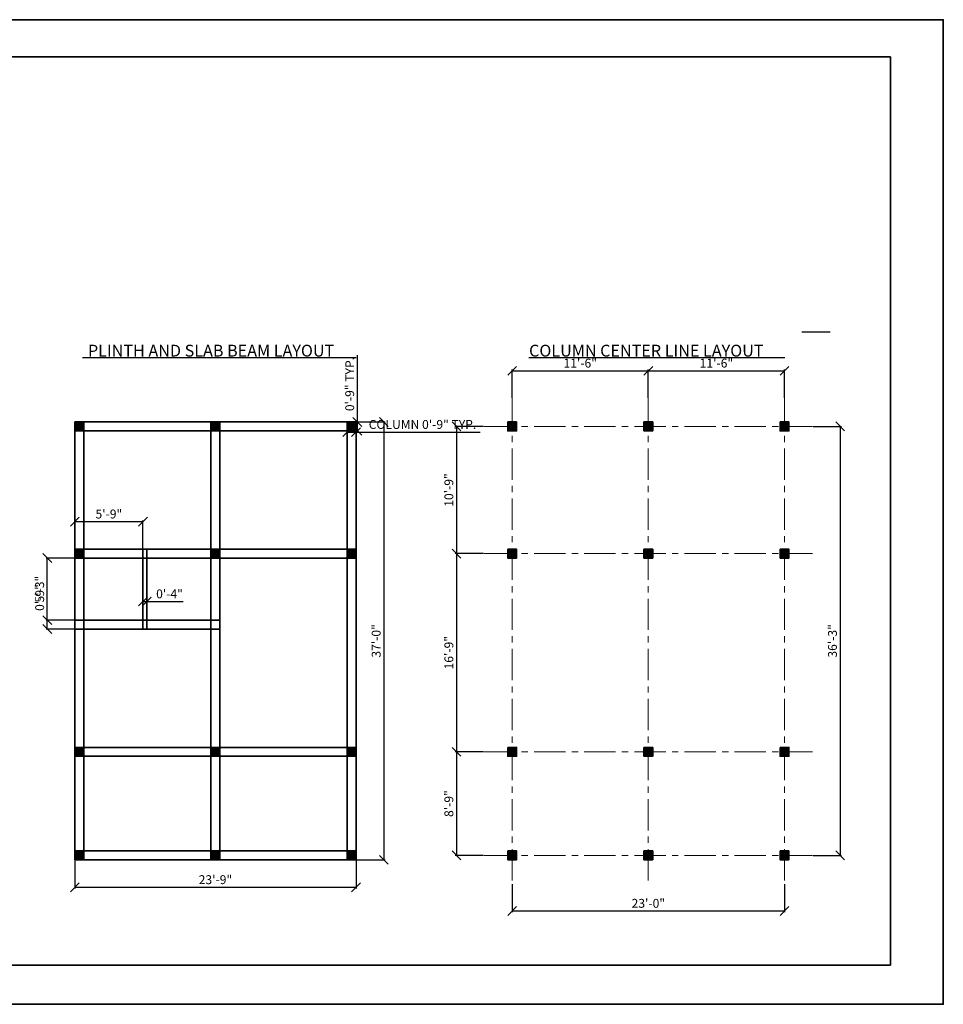
# Model space of a CAD drawing. Units: inches. Extents: x 1798 to 3594, y 1405 to 2404.
# Tile 6 of 6: x 2658 to 3594, y 1405 to 2404. Entities that reach past the tile are written whole.
import ezdxf

# ---------------------------------------------------------------- set-up
doc = ezdxf.new("R2010")
doc.units = ezdxf.units.IN
doc.linetypes.add('CENTER', pattern=[50.8, 31.75, -6.35, 6.35, -6.35])
for name, color, linetype, lineweight in [('A-ANNO-DIMS', 6, 'Continuous', 18), ('A-ANNO-TITL', 6, 'Continuous', 25), ('A-ANNO-TTLB', 7, 'Continuous', 35), ('S-BEAM', 7, 'Continuous', 35), ('S-COLS', 1, 'Continuous', 35), ('S-GRID', 8, 'CENTER', 13)]:
    doc.layers.add(name, color=color, linetype=linetype, lineweight=lineweight)
doc.styles.get("Standard").update_dxf_attribs({"font": 'arial.ttf'})
doc.dimstyles.new('ISO-25', dxfattribs={"dimtxt": 9, "dimasz": 9, "dimexe": 1.25, "dimexo": 0.625, "dimgap": 2, "dimtad": 1, "dimdec": 1, "dimlunit": 4, "dimtxsty": 'Standard', "dimblk": 'OBLIQUE', "dimcen": 2.5, "dimazin": 0, "dimtfac": 1, "dimtdec": 1, "dimtmove": 0, "dimatfit": 3, "dimfxl": 1, "dimarcsym": 0})

# ---------------------------------------------------------------- blocks, each defined once
blk = doc.blocks.new('COLUMN-9X9')
h = blk.add_hatch(color=256)
h.dxf.hatch_style = 1
h.paths.add_polyline_path([(9, 9), (0, 9), (0, 0), (9, 0)])
blk.add_lwpolyline([(0, 9), (9, 9), (9, 0), (0, 0)], close=True)
blk = doc.blocks.new('_Oblique')
at = {"color": 0, "linetype": 'ByBlock', "lineweight": -2}
blk.add_line((-0.5, -0.5), (0.5, 0.5), dxfattribs=at)
blk = doc.blocks.new('*D13')
at = {"layer": 'A-ANNO-DIMS', "color": 0, "lineweight": -2, "transparency": 16777216}
for p, q in [((2990.01, 1986.19), (2990.01, 1984.21)), ((2990.01, 1985.46), (2999.01, 1985.46)), ((2999.01, 1986.19), (2999.01, 1984.21)), ((2999.01, 1985.46), (3124.75, 1985.46))]:
    blk.add_line(p, q, dxfattribs=at)
at = {"layer": 'Defpoints', "color": 0, "transparency": 16777216}
for p in [(2990.01, 1986.81), (2999.01, 1986.81), (2999.01, 1985.46)]:
    blk.add_point(p, dxfattribs=at)
at = {"layer": 'A-ANNO-DIMS', "color": 0, "lineweight": -2, "transparency": 16777216, "xscale": 9, "yscale": 9, "zscale": 9, "rotation": 180}
blk.add_blockref('_Oblique', (2990.01, 1985.46), dxfattribs=at)
at = {"layer": 'A-ANNO-DIMS', "color": 0, "lineweight": -2, "transparency": 16777216, "xscale": 9, "yscale": 9, "zscale": 9}
blk.add_blockref('_Oblique', (2999.01, 1985.46), dxfattribs=at)
at = {"layer": 'A-ANNO-DIMS', "color": 0, "transparency": 16777216, "insert": (3066.38, 1992.12), "char_height": 9, "attachment_point": 5}
blk.add_mtext('COLUMN 0\'-9" TYP.', dxfattribs=at)
blk = doc.blocks.new('*D14')
at = {"layer": 'A-ANNO-DIMS', "color": 0, "lineweight": -2, "transparency": 16777216}
for p, q in [((3000.36, 1995.81), (3000.36, 2063.67)), ((2999.64, 1995.81), (3001.61, 1995.81)), ((3000.36, 1986.81), (3000.36, 1995.81)), ((2999.64, 1986.81), (3001.61, 1986.81))]:
    blk.add_line(p, q, dxfattribs=at)
at = {"layer": 'Defpoints', "color": 0, "transparency": 16777216}
for p in [(2999.01, 1995.81), (3000.36, 1995.81), (2999.01, 1986.81)]:
    blk.add_point(p, dxfattribs=at)
at = {"layer": 'A-ANNO-DIMS', "color": 0, "lineweight": -2, "transparency": 16777216, "xscale": 9, "yscale": 9, "zscale": 9}
for p, rotation in [((3000.36, 1995.81), 90), ((3000.36, 1986.81), 270)]:
    blk.add_blockref('_Oblique', p, dxfattribs=dict(at, rotation=rotation))
at = {"layer": 'A-ANNO-DIMS', "color": 0, "transparency": 16777216, "insert": (2993.77, 2034.24), "char_height": 9, "attachment_point": 5, "rotation": 90}
blk.add_mtext('0\'-9" TYP.', dxfattribs=at)
blk = doc.blocks.new('*D66')
at = {"layer": 'A-ANNO-DIMS', "color": 0, "lineweight": -2, "transparency": 16777216}
for p, q in [((2714.01, 1551.19), (2714.01, 1522.66)), ((2999.01, 1551.19), (2999.01, 1522.66)), ((2714.01, 1523.91), (2999.01, 1523.91))]:
    blk.add_line(p, q, dxfattribs=at)
at = {"layer": 'Defpoints', "color": 0, "transparency": 16777216}
for p in [(2714.01, 1551.81), (2999.01, 1551.81), (2999.01, 1523.91)]:
    blk.add_point(p, dxfattribs=at)
at = {"layer": 'A-ANNO-DIMS', "color": 0, "lineweight": -2, "transparency": 16777216, "xscale": 9, "yscale": 9, "zscale": 9, "rotation": 180}
blk.add_blockref('_Oblique', (2714.01, 1523.91), dxfattribs=at)
at = {"layer": 'A-ANNO-DIMS', "color": 0, "lineweight": -2, "transparency": 16777216, "xscale": 9, "yscale": 9, "zscale": 9}
blk.add_blockref('_Oblique', (2999.01, 1523.91), dxfattribs=at)
at = {"layer": 'A-ANNO-DIMS', "color": 0, "transparency": 16777216, "insert": (2856.51, 1530.51), "char_height": 9, "attachment_point": 5}
blk.add_mtext('23\'-9"', dxfattribs=at)
blk = doc.blocks.new('*D67')
at = {"layer": 'A-ANNO-DIMS', "color": 0, "lineweight": -2, "transparency": 16777216}
for p, q in [((2999.64, 1995.81), (3028.44, 1995.81)), ((3027.19, 1995.81), (3027.19, 1551.81)), ((2999.64, 1551.81), (3028.44, 1551.81))]:
    blk.add_line(p, q, dxfattribs=at)
at = {"layer": 'Defpoints', "color": 0, "transparency": 16777216}
for p in [(2999.01, 1995.81), (2999.01, 1551.81), (3027.19, 1551.81)]:
    blk.add_point(p, dxfattribs=at)
at = {"layer": 'A-ANNO-DIMS', "color": 0, "lineweight": -2, "transparency": 16777216, "xscale": 9, "yscale": 9, "zscale": 9}
for p, rotation in [((3027.19, 1995.81), 90), ((3027.19, 1551.81), 270)]:
    blk.add_blockref('_Oblique', p, dxfattribs=dict(at, rotation=rotation))
at = {"layer": 'A-ANNO-DIMS', "color": 0, "transparency": 16777216, "insert": (3020.6, 1773.81), "char_height": 9, "attachment_point": 5, "rotation": 90}
blk.add_mtext('37\'-0"', dxfattribs=at)
blk = doc.blocks.new('*D68')
at = {"layer": 'A-ANNO-DIMS', "color": 0, "lineweight": -2, "transparency": 16777216}
for p, q in [((2714.01, 1867.44), (2714.01, 1895.96)), ((2714.01, 1894.71), (2783.01, 1894.71)), ((2783.01, 1867.44), (2783.01, 1895.96))]:
    blk.add_line(p, q, dxfattribs=at)
at = {"layer": 'Defpoints', "color": 0, "transparency": 16777216}
for p in [(2783.01, 1894.71), (2714.01, 1866.81), (2783.01, 1866.81)]:
    blk.add_point(p, dxfattribs=at)
at = {"layer": 'A-ANNO-DIMS', "color": 0, "lineweight": -2, "transparency": 16777216, "xscale": 9, "yscale": 9, "zscale": 9, "rotation": 180}
blk.add_blockref('_Oblique', (2714.01, 1894.71), dxfattribs=at)
at = {"layer": 'A-ANNO-DIMS', "color": 0, "lineweight": -2, "transparency": 16777216, "xscale": 9, "yscale": 9, "zscale": 9}
blk.add_blockref('_Oblique', (2783.01, 1894.71), dxfattribs=at)
at = {"layer": 'A-ANNO-DIMS', "color": 0, "transparency": 16777216, "insert": (2748.51, 1901.31), "char_height": 9, "attachment_point": 5}
blk.add_mtext('5\'-9"', dxfattribs=at)
blk = doc.blocks.new('*D69')
at = {"layer": 'A-ANNO-DIMS', "color": 0, "lineweight": -2, "transparency": 16777216}
for p, q in [((2783.01, 1786.44), (2783.01, 1814.96)), ((2783.01, 1813.71), (2787.01, 1813.71)), ((2787.01, 1786.44), (2787.01, 1814.96)), ((2787.01, 1813.71), (2823.94, 1813.71))]:
    blk.add_line(p, q, dxfattribs=at)
at = {"layer": 'Defpoints', "color": 0, "transparency": 16777216}
for p in [(2787.01, 1813.71), (2783.01, 1785.81), (2787.01, 1785.81)]:
    blk.add_point(p, dxfattribs=at)
at = {"layer": 'A-ANNO-DIMS', "color": 0, "lineweight": -2, "transparency": 16777216, "xscale": 9, "yscale": 9, "zscale": 9, "rotation": 180}
blk.add_blockref('_Oblique', (2783.01, 1813.71), dxfattribs=at)
at = {"layer": 'A-ANNO-DIMS', "color": 0, "lineweight": -2, "transparency": 16777216, "xscale": 9, "yscale": 9, "zscale": 9}
blk.add_blockref('_Oblique', (2787.01, 1813.71), dxfattribs=at)
at = {"layer": 'A-ANNO-DIMS', "color": 0, "transparency": 16777216, "insert": (2809.98, 1820.31), "char_height": 9, "attachment_point": 5}
blk.add_mtext('0\'-4"', dxfattribs=at)
blk = doc.blocks.new('*D70')
at = {"layer": 'A-ANNO-DIMS', "color": 0, "lineweight": -2, "transparency": 16777216}
for p, q in [((2713.39, 1857.81), (2684.86, 1857.81)), ((2686.11, 1794.81), (2686.11, 1857.81)), ((2713.39, 1794.81), (2684.86, 1794.81))]:
    blk.add_line(p, q, dxfattribs=at)
at = {"layer": 'Defpoints', "color": 0, "transparency": 16777216}
for p in [(2686.11, 1857.81), (2714.01, 1857.81), (2714.01, 1794.81)]:
    blk.add_point(p, dxfattribs=at)
at = {"layer": 'A-ANNO-DIMS', "color": 0, "lineweight": -2, "transparency": 16777216, "xscale": 9, "yscale": 9, "zscale": 9}
for p, rotation in [((2686.11, 1857.81), 90), ((2686.11, 1794.81), 270)]:
    blk.add_blockref('_Oblique', p, dxfattribs=dict(at, rotation=rotation))
at = {"layer": 'A-ANNO-DIMS', "color": 0, "transparency": 16777216, "insert": (2679.51, 1826.31), "char_height": 9, "attachment_point": 5, "rotation": 90}
blk.add_mtext('5\'-3"', dxfattribs=at)
blk = doc.blocks.new('*D71')
at = {"layer": 'A-ANNO-DIMS', "color": 0, "lineweight": -2, "transparency": 16777216}
for p, q in [((2686.11, 1794.81), (2686.11, 1831.74)), ((2713.39, 1794.81), (2684.86, 1794.81)), ((2686.11, 1785.81), (2686.11, 1794.81)), ((2713.39, 1785.81), (2684.86, 1785.81))]:
    blk.add_line(p, q, dxfattribs=at)
at = {"layer": 'Defpoints', "color": 0, "transparency": 16777216}
for p in [(2686.11, 1794.81), (2714.01, 1794.81), (2714.01, 1785.81)]:
    blk.add_point(p, dxfattribs=at)
at = {"layer": 'A-ANNO-DIMS', "color": 0, "lineweight": -2, "transparency": 16777216, "xscale": 9, "yscale": 9, "zscale": 9}
for p, rotation in [((2686.11, 1794.81), 90), ((2686.11, 1785.81), 270)]:
    blk.add_blockref('_Oblique', p, dxfattribs=dict(at, rotation=rotation))
at = {"layer": 'A-ANNO-DIMS', "color": 0, "transparency": 16777216, "insert": (2679.52, 1817.77), "char_height": 9, "attachment_point": 5, "rotation": 90}
blk.add_mtext('0\'-9"', dxfattribs=at)
blk = doc.blocks.new('*D72')
at = {"layer": 'A-ANNO-DIMS', "color": 0, "lineweight": -2, "transparency": 16777216}
for p, q in [((3157.27, 2020.44), (3157.27, 2048.96)), ((3157.27, 2047.71), (3295.27, 2047.71)), ((3295.27, 2020.44), (3295.27, 2048.96))]:
    blk.add_line(p, q, dxfattribs=at)
at = {"layer": 'Defpoints', "color": 0, "transparency": 16777216}
for p in [(3295.27, 2047.71), (3157.27, 2019.81), (3295.27, 2019.81)]:
    blk.add_point(p, dxfattribs=at)
at = {"layer": 'A-ANNO-DIMS', "color": 0, "lineweight": -2, "transparency": 16777216, "xscale": 9, "yscale": 9, "zscale": 9, "rotation": 180}
blk.add_blockref('_Oblique', (3157.27, 2047.71), dxfattribs=at)
at = {"layer": 'A-ANNO-DIMS', "color": 0, "lineweight": -2, "transparency": 16777216, "xscale": 9, "yscale": 9, "zscale": 9}
blk.add_blockref('_Oblique', (3295.27, 2047.71), dxfattribs=at)
at = {"layer": 'A-ANNO-DIMS', "color": 0, "transparency": 16777216, "insert": (3226.27, 2054.31), "char_height": 9, "attachment_point": 5}
blk.add_mtext('11\'-6"', dxfattribs=at)
blk = doc.blocks.new('*D73')
at = {"layer": 'A-ANNO-DIMS', "color": 0, "lineweight": -2, "transparency": 16777216}
for p, q in [((3295.27, 2020.44), (3295.27, 2048.96)), ((3295.27, 2047.71), (3433.27, 2047.71)), ((3433.27, 2020.44), (3433.27, 2048.96))]:
    blk.add_line(p, q, dxfattribs=at)
at = {"layer": 'Defpoints', "color": 0, "transparency": 16777216}
for p in [(3433.27, 2047.71), (3295.27, 2019.81), (3433.27, 2019.81)]:
    blk.add_point(p, dxfattribs=at)
at = {"layer": 'A-ANNO-DIMS', "color": 0, "lineweight": -2, "transparency": 16777216, "xscale": 9, "yscale": 9, "zscale": 9, "rotation": 180}
blk.add_blockref('_Oblique', (3295.27, 2047.71), dxfattribs=at)
at = {"layer": 'A-ANNO-DIMS', "color": 0, "lineweight": -2, "transparency": 16777216, "xscale": 9, "yscale": 9, "zscale": 9}
blk.add_blockref('_Oblique', (3433.27, 2047.71), dxfattribs=at)
at = {"layer": 'A-ANNO-DIMS', "color": 0, "transparency": 16777216, "insert": (3364.27, 2054.31), "char_height": 9, "attachment_point": 5}
blk.add_mtext('11\'-6"', dxfattribs=at)
blk = doc.blocks.new('*D74')
at = {"layer": 'A-ANNO-DIMS', "color": 0, "lineweight": -2, "transparency": 16777216}
for p, q in [((3157.27, 1527.19), (3157.27, 1498.66)), ((3433.27, 1527.19), (3433.27, 1498.66)), ((3157.27, 1499.91), (3433.27, 1499.91))]:
    blk.add_line(p, q, dxfattribs=at)
at = {"layer": 'Defpoints', "color": 0, "transparency": 16777216}
for p in [(3157.27, 1527.81), (3433.27, 1527.81), (3433.27, 1499.91)]:
    blk.add_point(p, dxfattribs=at)
at = {"layer": 'A-ANNO-DIMS', "color": 0, "lineweight": -2, "transparency": 16777216, "xscale": 9, "yscale": 9, "zscale": 9, "rotation": 180}
blk.add_blockref('_Oblique', (3157.27, 1499.91), dxfattribs=at)
at = {"layer": 'A-ANNO-DIMS', "color": 0, "lineweight": -2, "transparency": 16777216, "xscale": 9, "yscale": 9, "zscale": 9}
blk.add_blockref('_Oblique', (3433.27, 1499.91), dxfattribs=at)
at = {"layer": 'A-ANNO-DIMS', "color": 0, "transparency": 16777216, "insert": (3295.27, 1506.51), "char_height": 9, "attachment_point": 5}
blk.add_mtext('23\'-0"', dxfattribs=at)
blk = doc.blocks.new('*D75')
at = {"layer": 'A-ANNO-DIMS', "color": 0, "lineweight": -2, "transparency": 16777216}
for p, q in [((3128.14, 1991.31), (3099.62, 1991.31)), ((3100.87, 1991.31), (3100.87, 1862.31)), ((3128.14, 1862.31), (3099.62, 1862.31))]:
    blk.add_line(p, q, dxfattribs=at)
at = {"layer": 'Defpoints', "color": 0, "transparency": 16777216}
for p in [(3128.77, 1991.31), (3100.87, 1862.31), (3128.77, 1862.31)]:
    blk.add_point(p, dxfattribs=at)
at = {"layer": 'A-ANNO-DIMS', "color": 0, "lineweight": -2, "transparency": 16777216, "xscale": 9, "yscale": 9, "zscale": 9}
for p, rotation in [((3100.87, 1991.31), 90), ((3100.87, 1862.31), 270)]:
    blk.add_blockref('_Oblique', p, dxfattribs=dict(at, rotation=rotation))
at = {"layer": 'A-ANNO-DIMS', "color": 0, "transparency": 16777216, "insert": (3094.27, 1926.81), "char_height": 9, "attachment_point": 5, "rotation": 90}
blk.add_mtext('10\'-9"', dxfattribs=at)
blk = doc.blocks.new('*D76')
at = {"layer": 'A-ANNO-DIMS', "color": 0, "lineweight": -2, "transparency": 16777216}
for p, q in [((3128.14, 1862.31), (3099.62, 1862.31)), ((3100.87, 1862.31), (3100.87, 1661.31)), ((3128.14, 1661.31), (3099.62, 1661.31))]:
    blk.add_line(p, q, dxfattribs=at)
at = {"layer": 'Defpoints', "color": 0, "transparency": 16777216}
for p in [(3128.77, 1862.31), (3100.87, 1661.31), (3128.77, 1661.31)]:
    blk.add_point(p, dxfattribs=at)
at = {"layer": 'A-ANNO-DIMS', "color": 0, "lineweight": -2, "transparency": 16777216, "xscale": 9, "yscale": 9, "zscale": 9}
for p, rotation in [((3100.87, 1862.31), 90), ((3100.87, 1661.31), 270)]:
    blk.add_blockref('_Oblique', p, dxfattribs=dict(at, rotation=rotation))
at = {"layer": 'A-ANNO-DIMS', "color": 0, "transparency": 16777216, "insert": (3094.27, 1761.81), "char_height": 9, "attachment_point": 5, "rotation": 90}
blk.add_mtext('16\'-9"', dxfattribs=at)
blk = doc.blocks.new('*D77')
at = {"layer": 'A-ANNO-DIMS', "color": 0, "lineweight": -2, "transparency": 16777216}
for p, q in [((3128.14, 1661.31), (3099.62, 1661.31)), ((3100.87, 1661.31), (3100.87, 1556.31)), ((3128.14, 1556.31), (3099.62, 1556.31))]:
    blk.add_line(p, q, dxfattribs=at)
at = {"layer": 'Defpoints', "color": 0, "transparency": 16777216}
for p in [(3128.77, 1661.31), (3100.87, 1556.31), (3128.77, 1556.31)]:
    blk.add_point(p, dxfattribs=at)
at = {"layer": 'A-ANNO-DIMS', "color": 0, "lineweight": -2, "transparency": 16777216, "xscale": 9, "yscale": 9, "zscale": 9}
for p, rotation in [((3100.87, 1661.31), 90), ((3100.87, 1556.31), 270)]:
    blk.add_blockref('_Oblique', p, dxfattribs=dict(at, rotation=rotation))
at = {"layer": 'A-ANNO-DIMS', "color": 0, "transparency": 16777216, "insert": (3094.27, 1608.81), "char_height": 9, "attachment_point": 5, "rotation": 90}
blk.add_mtext('8\'-9"', dxfattribs=at)
blk = doc.blocks.new('*D78')
at = {"layer": 'A-ANNO-DIMS', "color": 0, "lineweight": -2, "transparency": 16777216}
for p, q in [((3462.39, 1991.31), (3490.92, 1991.31)), ((3489.67, 1991.31), (3489.67, 1556.31)), ((3462.39, 1556.31), (3490.92, 1556.31))]:
    blk.add_line(p, q, dxfattribs=at)
at = {"layer": 'Defpoints', "color": 0, "transparency": 16777216}
for p in [(3461.77, 1991.31), (3461.77, 1556.31), (3489.67, 1556.31)]:
    blk.add_point(p, dxfattribs=at)
at = {"layer": 'A-ANNO-DIMS', "color": 0, "lineweight": -2, "transparency": 16777216, "xscale": 9, "yscale": 9, "zscale": 9}
for p, rotation in [((3489.67, 1991.31), 90), ((3489.67, 1556.31), 270)]:
    blk.add_blockref('_Oblique', p, dxfattribs=dict(at, rotation=rotation))
at = {"layer": 'A-ANNO-DIMS', "color": 0, "transparency": 16777216, "insert": (3483.07, 1773.81), "char_height": 9, "attachment_point": 5, "rotation": 90}
blk.add_mtext('36\'-3"', dxfattribs=at)

msp = doc.modelspace()

# ---------------------------------------------------------------- linework, layer by layer
at = {"layer": 'A-ANNO-TITL'}
for p, q in [((3450.72, 2087.28), (3479.45, 2087.28)), ((2721.88, 2061.08), (2999.29, 2061.08)), ((3174.12, 2061.08), (3433.61, 2061.08))]:
    msp.add_line(p, q, dxfattribs=at)
at = {"layer": 'A-ANNO-TTLB'}
for points in [[(1798.35, 2403.73), (3594.23, 2403.73), (3594.23, 1405.28), (1798.35, 1405.28)], [(1855.68, 2366.05), (3540.6, 2366.05), (3540.6, 1444.98), (1855.68, 1444.98)]]:
    msp.add_lwpolyline(points, close=True, dxfattribs=at)
at = {"layer": 'S-BEAM'}
for p, q in [((2714.01, 1995.81), (2999.01, 1995.81)), ((2714.01, 1995.81), (2714.01, 1551.81)), ((2852.01, 1995.81), (2852.01, 1785.81)), ((2861.01, 1995.81), (2861.01, 1665.81)), ((2999.01, 1995.81), (2999.01, 1551.81)), ((2714.01, 1986.81), (2990.01, 1986.81)), ((2723.01, 1986.81), (2723.01, 1551.81)), ((2990.01, 1986.81), (2990.01, 1551.81)), ((2714.01, 1866.81), (2833.01, 1866.81)), ((2714.01, 1866.81), (2999.01, 1866.81)), ((2714.01, 1857.81), (2852.01, 1857.81)), ((2779.01, 1866.81), (2791.01, 1866.81)), ((2779.01, 1857.81), (2783.01, 1857.81)), ((2783.01, 1866.81), (2783.01, 1785.81)), ((2787.01, 1866.81), (2787.01, 1785.81)), ((2787.01, 1857.81), (2791.01, 1857.81)), ((2787.01, 1857.81), (2999.01, 1857.81)), ((2833.01, 1866.81), (2852.01, 1866.81)), ((2852.01, 1866.81), (2852.01, 1656.81)), ((2986.01, 1866.81), (2999.01, 1866.81)), ((2986.01, 1857.81), (2999.01, 1857.81)), ((2714.01, 1794.81), (2787.01, 1794.81)), ((2787.01, 1794.81), (2861.01, 1794.81)), ((2861.01, 1794.81), (2861.01, 1665.81)), ((2714.01, 1785.81), (2861.01, 1785.81)), ((2852.01, 1669.81), (2852.01, 1656.81)), ((2861.01, 1669.81), (2861.01, 1656.81)), ((2714.01, 1665.81), (2990.01, 1665.81)), ((2852.01, 1665.81), (2999.01, 1665.81)), ((2986.01, 1665.81), (2999.01, 1665.81)), ((2714.01, 1656.81), (2990.01, 1656.81)), ((2852.01, 1656.81), (2999.01, 1656.81)), ((2852.01, 1656.81), (2852.01, 1610.81)), ((2861.01, 1656.81), (2861.01, 1610.81)), ((2986.01, 1656.81), (2999.01, 1656.81)), ((2852.01, 1610.81), (2852.01, 1560.81)), ((2861.01, 1610.81), (2861.01, 1560.81)), ((2714.01, 1560.81), (2999.01, 1560.81)), ((2714.01, 1551.81), (2999.01, 1551.81))]:
    msp.add_line(p, q, dxfattribs=at)
at = {"layer": 'S-GRID'}
for p, q in [((3157.27, 2019.81), (3157.27, 1527.81)), ((3295.27, 2019.81), (3295.27, 1527.81)), ((3433.27, 2019.81), (3433.27, 1527.81)), ((3128.77, 1991.31), (3461.77, 1991.31)), ((3128.77, 1862.31), (3461.77, 1862.31)), ((3128.77, 1661.31), (3461.77, 1661.31)), ((3128.77, 1556.31), (3461.77, 1556.31))]:
    msp.add_line(p, q, dxfattribs=at)

# ---------------------------------------------------------------- block references
at = {"layer": 'S-COLS'}
for p in [(2714.01, 1986.81), (2852.01, 1986.81), (2990.01, 1986.81), (3152.77, 1986.81), (3290.77, 1986.81), (3428.77, 1986.81), (2714.01, 1857.81), (2852.01, 1857.81), (2990.01, 1857.81), (3152.77, 1857.81), (3290.77, 1857.81), (3428.77, 1857.81), (2714.01, 1656.81), (2852.01, 1656.81), (2990.01, 1656.81), (3152.77, 1656.81), (3290.77, 1656.81), (3428.77, 1656.81), (2714.01, 1551.81), (2852.01, 1551.81), (2990.01, 1551.81), (3152.77, 1551.81), (3290.77, 1551.81), (3428.77, 1551.81)]:
    msp.add_blockref('COLUMN-9X9', p, dxfattribs=at)

# ---------------------------------------------------------------- texts
at = {"layer": 'A-ANNO-TITL'}
for s, p in [('PLINTH AND SLAB BEAM LAYOUT', (2727.31, 2062.11)), ('COLUMN CENTER LINE LAYOUT', (3174.38, 2062.11))]:
    msp.add_text(s, height=12, dxfattribs=at).set_placement(p)

# ---------------------------------------------------------------- dimensions: what is measured, and where the dimension line sits
at = {"layer": 'A-ANNO-DIMS'}
dim = msp.add_linear_dim(base=(3000.36, 1995.81), p1=(2999.01, 1986.81), p2=(2999.01, 1995.81), angle=90, text='<> TYP.', dimstyle='ISO-25', override={"dimdec": 1, "dimlfac": 1, "dimrnd": 0, "dimzin": 1, "dimdsep": 46, "dimlunit": 4, "dimfrac": 2}, dxfattribs=at)
dim.commit()
dim.dimension.update_dxf_attribs({"geometry": '*D14', "text_midpoint": (2993.77, 2034.24)})
for base, p1, p2, picture, middle in [((3295.27, 2047.71), (3157.27, 2019.81), (3295.27, 2019.81), '*D72', (3226.27, 2054.31)), ((3433.27, 2047.71), (3295.27, 2019.81), (3433.27, 2019.81), '*D73', (3364.27, 2054.31)), ((2783.01, 1894.71), (2714.01, 1866.81), (2783.01, 1866.81), '*D68', (2748.51, 1901.31)), ((2999.01, 1523.91), (2714.01, 1551.81), (2999.01, 1551.81), '*D66', (2856.51, 1530.51)), ((3433.27, 1499.91), (3157.27, 1527.81), (3433.27, 1527.81), '*D74', (3295.27, 1506.51))]:
    dim = msp.add_linear_dim(base=base, p1=p1, p2=p2, dimstyle='ISO-25', override={"dimdec": 1, "dimlfac": 1, "dimrnd": 0, "dimzin": 1, "dimdsep": 46, "dimlunit": 4, "dimfrac": 2}, dxfattribs=at)
    dim.commit()
    dim.dimension.update_dxf_attribs({"geometry": picture, "text_midpoint": middle})
dim = msp.add_linear_dim(base=(2999.01, 1985.46), p1=(2990.01, 1986.81), p2=(2999.01, 1986.81), text='COLUMN <> TYP.', dimstyle='ISO-25', override={"dimdec": 1, "dimlfac": 1, "dimrnd": 0, "dimzin": 1, "dimdsep": 46, "dimlunit": 4, "dimfrac": 2}, dxfattribs=at)
dim.commit()
dim.dimension.update_dxf_attribs({"geometry": '*D13', "text_midpoint": (3066.38, 1992.12)})
for base, p1, p2, angle, picture, middle in [((3027.19, 1551.81), (2999.01, 1995.81), (2999.01, 1551.81), 90, '*D67', (3020.6, 1773.81)), ((3100.87, 1862.31), (3128.77, 1991.31), (3128.77, 1862.31), 90, '*D75', (3094.27, 1926.81)), ((3489.67, 1556.31), (3461.77, 1991.31), (3461.77, 1556.31), 90, '*D78', (3483.07, 1773.81)), ((2686.11, 1857.81), (2714.01, 1794.81), (2714.01, 1857.81), 90, '*D70', (2679.51, 1826.31)), ((3100.87, 1661.31), (3128.77, 1862.31), (3128.77, 1661.31), 90, '*D76', (3094.27, 1761.81)), ((2686.11, 1794.81), (2714.01, 1785.81), (2714.01, 1794.81), 90, '*D71', (2679.52, 1817.77)), ((2787.01, 1813.71), (2783.01, 1785.81), (2787.01, 1785.81), 0, '*D69', (2809.98, 1820.31)), ((3100.87, 1556.31), (3128.77, 1661.31), (3128.77, 1556.31), 90, '*D77', (3094.27, 1608.81))]:
    dim = msp.add_linear_dim(base=base, p1=p1, p2=p2, angle=angle, dimstyle='ISO-25', override={"dimdec": 1, "dimlfac": 1, "dimrnd": 0, "dimzin": 1, "dimdsep": 46, "dimlunit": 4, "dimfrac": 2}, dxfattribs=at)
    dim.commit()
    dim.dimension.update_dxf_attribs({"geometry": picture, "text_midpoint": middle})

doc.saveas('drawing.dxf')
